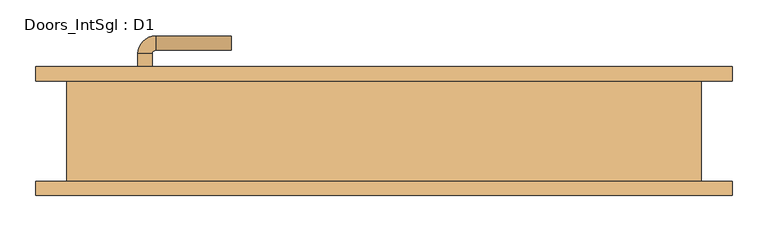
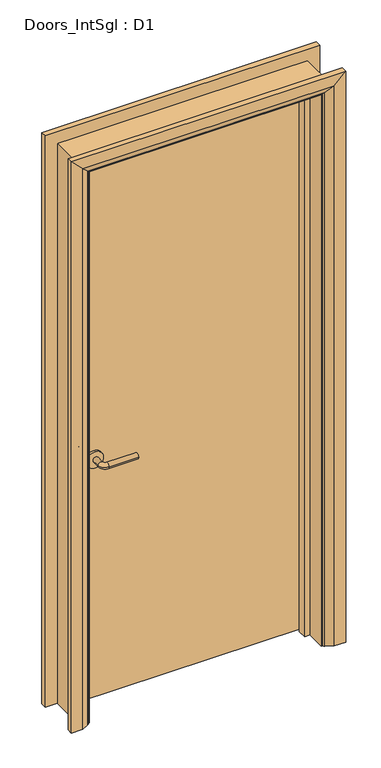
"""IFC4 building model written with IfcOpenShell, lengths in millimetres: door geometry, Doors_IntSgl : D1."""

from ifc_helpers import new_model, si_unit, point, frame, frame_2d, origin, place, context, project, spatial, polyline, circle_curve, ellipse_curve, trimmed, segment, composite_curve, outline, extrude, faceted_brep, source, transform, mapped, element, save
from ifc_brep_helpers import plane_surface, cylinder_surface, revolved_surface, advanced_brep


def doors_intsgl_d1_9c7e8c97(model_context):
    return source(origin(), model_context, "Body", "SolidModel", [
        advanced_brep(
        [(-343.0, 24.0, 900.0), (-323.0, 24.0, 900.0), (-323.0, -6.0, 900.0), (-343.0, -6.0, 900.0), (-318.0, -11.0, 900.0), (-318.0, -31.0, 900.0), (-213.0, -31.0, 900.0), (-213.0, -11.0, 900.0)],
        [
            (0, 1, circle_curve(frame((-333.0, 24.0, 900.0), z_axis=(0.0, 1.0, 0.0), x_axis=(1.0, 0.0, 0.0)), 10.0)),
            (1, 0, circle_curve(frame((-333.0, 24.0, 900.0), z_axis=(0.0, 1.0, 0.0), x_axis=(1.0, 0.0, 0.0)), 10.0)),
            (1, 2),
            (2, 3, circle_curve(frame((-333.0, -6.0, 900.0), z_axis=(0.0, 1.0, 0.0), x_axis=(1.0, 0.0, 0.0)), 10.0)),
            (3, 0),
            (3, 2, circle_curve(frame((-333.0, -6.0, 900.0), z_axis=(0.0, 1.0, 0.0), x_axis=(1.0, 0.0, 0.0)), 10.0)),
            (4, 5, circle_curve(frame((-318.0, -21.0, 900.0), z_axis=(-1.0, 0.0, 0.0), x_axis=(0.0, 1.0, 0.0)), 10.0)),
            (5, 3, circle_curve(frame((-318.0, -6.0, 900.0), z_axis=(0.0, 0.0, -1.0), x_axis=(-1.0, 0.0, 0.0)), 25.0)),
            (2, 4, circle_curve(frame((-318.0, -6.0, 900.0), z_axis=(0.0, 0.0, 1.0), x_axis=(-1.0, 0.0, 0.0)), 5.0)),
            (5, 4, circle_curve(frame((-318.0, -21.0, 900.0), z_axis=(-1.0, 0.0, 0.0), x_axis=(0.0, 1.0, 0.0)), 10.0)),
            (6, 7, circle_curve(frame((-213.0, -21.0, 900.0), z_axis=(1.0, 0.0, 0.0), x_axis=(0.0, 1.0, 0.0)), 10.0)),
            (7, 6, circle_curve(frame((-213.0, -21.0, 900.0), z_axis=(1.0, 0.0, 0.0), x_axis=(0.0, 1.0, 0.0)), 10.0)),
            (4, 7),
            (6, 5),
        ],
        [
            plane_surface(frame((-333.0, 24.0, 900.0), z_axis=(0.0, 1.0, 0.0), x_axis=(0.0, 0.0, 1.0))),
            cylinder_surface(frame((-333.0, 24.0, 900.0), z_axis=(0.0, 1.0, 0.0), x_axis=(1.0, 0.0, 0.0)), 10.0),
            revolved_surface(trimmed(ellipse_curve(frame((-333.0, -6.0, 900.0), z_axis=(0.0, -1.0, 0.0), x_axis=(1.0, 0.0, 0.0)), 10.0, 10.0), [point((-343.0, -6.0, 900.0))], [point((-323.0, -6.0, 900.0))], True, "CARTESIAN"), (-318.0, -6.0, 900.0), (0.0, 0.0, -1.0)),
            revolved_surface(trimmed(ellipse_curve(frame((-333.0, -6.0, 900.0), z_axis=(0.0, -1.0, 0.0), x_axis=(1.0, 0.0, 0.0)), 10.0, 10.0), [point((-323.0, -6.0, 900.0))], [point((-343.0, -6.0, 900.0))], True, "CARTESIAN"), (-318.0, -6.0, 900.0), (0.0, 0.0, -1.0)),
            plane_surface(frame((-213.0, -21.0, 900.0), z_axis=(1.0, 0.0, 0.0), x_axis=(0.0, 0.0, 1.0))),
            cylinder_surface(frame((-318.0, -21.0, 900.0), z_axis=(-1.0, 0.0, 0.0), x_axis=(0.0, 1.0, 0.0)), 10.0),
        ],
        [
            (0, [[1, 2]]),
            (1, [[3, 4, 5, -2]]),
            (1, [[-5, 6, -3, -1]]),
            (2, [[7, 8, -4, 9]]),
            (3, [[10, -9, -6, -8]]),
            (4, [[11, 12]]),
            (5, [[13, -11, 14, -7]]),
            (5, [[-14, -12, -13, -10]]),
        ],
    ),
        extrude(outline(composite_curve([segment(trimmed(circle_curve(frame_2d((900.0, -335.5)), 30.0), [point((900.0, -365.5))], [point((900.0, -305.5))], False, "CARTESIAN"), True, "CONTINUOUS"), segment(trimmed(circle_curve(frame_2d((900.0, -335.5)), 30.0), [point((900.0, -305.5))], [point((900.0, -365.5))], False, "CARTESIAN"), True, "CONTINUOUS")], self_intersect=False)), frame((0.0, 24.0, 0.0), z_axis=(0.0, 1.0, 0.0), x_axis=(0.0, 0.0, 1.0)), (0.0, 0.0, 1.0), 8.0),
        advanced_brep(
        [(-343.0, 78.0, 900.0), (-323.0, 78.0, 900.0), (-343.0, 108.0, 900.0), (-323.0, 108.0, 900.0), (-318.0, 113.0, 900.0), (-318.0, 133.0, 900.0), (-213.0, 133.0, 900.0), (-213.0, 113.0, 900.0)],
        [
            (0, 1, circle_curve(frame((-333.0, 78.0, 900.0), z_axis=(0.0, -1.0, 0.0), x_axis=(1.0, 0.0, 0.0)), 10.0)),
            (1, 0, circle_curve(frame((-333.0, 78.0, 900.0), z_axis=(0.0, -1.0, 0.0), x_axis=(1.0, 0.0, 0.0)), 10.0)),
            (0, 2),
            (2, 3, circle_curve(frame((-333.0, 108.0, 900.0), z_axis=(0.0, -1.0, 0.0), x_axis=(1.0, 0.0, 0.0)), 10.0)),
            (3, 1),
            (3, 2, circle_curve(frame((-333.0, 108.0, 900.0), z_axis=(0.0, -1.0, 0.0), x_axis=(1.0, 0.0, 0.0)), 10.0)),
            (4, 3, circle_curve(frame((-318.0, 108.0, 900.0), z_axis=(0.0, 0.0, 1.0), x_axis=(-1.0, 0.0, 0.0)), 5.0)),
            (2, 5, circle_curve(frame((-318.0, 108.0, 900.0), z_axis=(0.0, 0.0, -1.0), x_axis=(-1.0, 0.0, 0.0)), 25.0)),
            (5, 4, circle_curve(frame((-318.0, 123.0, 900.0), z_axis=(-1.0, 0.0, 0.0), x_axis=(0.0, -1.0, 0.0)), 10.0)),
            (4, 5, circle_curve(frame((-318.0, 123.0, 900.0), z_axis=(-1.0, 0.0, 0.0), x_axis=(0.0, -1.0, 0.0)), 10.0)),
            (6, 7, circle_curve(frame((-213.0, 123.0, 900.0), z_axis=(1.0, 0.0, 0.0), x_axis=(0.0, -1.0, 0.0)), 10.0)),
            (7, 6, circle_curve(frame((-213.0, 123.0, 900.0), z_axis=(1.0, 0.0, 0.0), x_axis=(0.0, -1.0, 0.0)), 10.0)),
            (5, 6),
            (7, 4),
        ],
        [
            plane_surface(frame((-333.0, 78.0, 900.0), z_axis=(0.0, -1.0, 0.0), x_axis=(0.0, 0.0, 1.0))),
            cylinder_surface(frame((-333.0, 78.0, 900.0), z_axis=(0.0, -1.0, 0.0), x_axis=(1.0, 0.0, 0.0)), 10.0),
            revolved_surface(trimmed(ellipse_curve(frame((-333.0, 108.0, 900.0), z_axis=(0.0, -1.0, 0.0), x_axis=(1.0, 0.0, 0.0)), 10.0, 10.0), [point((-343.0, 108.0, 900.0))], [point((-323.0, 108.0, 900.0))], True, "CARTESIAN"), (-318.0, 108.0, 900.0), (0.0, 0.0, -1.0)),
            revolved_surface(trimmed(ellipse_curve(frame((-333.0, 108.0, 900.0), z_axis=(0.0, -1.0, 0.0), x_axis=(1.0, 0.0, 0.0)), 10.0, 10.0), [point((-323.0, 108.0, 900.0))], [point((-343.0, 108.0, 900.0))], True, "CARTESIAN"), (-318.0, 108.0, 900.0), (0.0, 0.0, -1.0)),
            plane_surface(frame((-213.0, 123.0, 900.0), z_axis=(1.0, 0.0, 0.0), x_axis=(0.0, 0.0, 1.0))),
            cylinder_surface(frame((-318.0, 123.0, 900.0), z_axis=(-1.0, 0.0, 0.0), x_axis=(0.0, -1.0, 0.0)), 10.0),
        ],
        [
            (0, [[1, 2]]),
            (1, [[-1, 3, 4, 5]]),
            (1, [[-2, -5, 6, -3]]),
            (2, [[7, -4, 8, 9]]),
            (3, [[-8, -6, -7, 10]]),
            (4, [[11, 12]]),
            (5, [[-9, 13, -12, 14]]),
            (5, [[-10, -14, -11, -13]]),
        ],
    ),
        extrude(outline(composite_curve([segment(trimmed(circle_curve(frame_2d((900.0, -335.5)), 30.0), [point((900.0, -365.5))], [point((900.0, -305.5))], False, "CARTESIAN"), True, "CONTINUOUS"), segment(trimmed(circle_curve(frame_2d((900.0, -335.5)), 30.0), [point((900.0, -305.5))], [point((900.0, -365.5))], False, "CARTESIAN"), True, "CONTINUOUS")], self_intersect=False)), frame((0.0, 70.0, 0.0), z_axis=(0.0, 1.0, 0.0), x_axis=(0.0, 0.0, 1.0)), (0.0, 0.0, 1.0), 8.0),
        extrude(outline(polyline([(408.0, 32.0), (-408.0, 32.0), (-408.0, 70.0), (408.0, 70.0), (408.0, 32.0)])), frame((0.0, 0.0, 8.0), z_axis=(0.0, 0.0, 1.0), x_axis=(1.0, 0.0, 0.0)), (0.0, 0.0, 1.0), 2050.0),
        advanced_brep(
        [(485.0, 90.0, 0.0), (485.0, 70.0, 0.0), (415.0, 70.0, 0.0), (419.0, 76.0, 0.0), (445.0, 90.0, 0.0), (485.0, 90.0, 2135.0), (485.0, 70.0, 2135.0), (-485.0, 70.0, 2135.0), (-485.0, 70.0, 0.0), (-415.0, 70.0, 0.0), (-415.0, 70.0, 2065.0), (415.0, 70.0, 2065.0), (419.0, 76.0, 2069.0), (445.0, 90.0, 2095.0), (-445.0, 90.0, 2095.0), (-445.0, 90.0, 0.0), (-485.0, 90.0, 0.0), (-485.0, 90.0, 2135.0), (-419.0, 76.0, 0.0), (-419.0, 76.0, 2069.0)],
        [
            (0, 1),
            (1, 2),
            (2, 3, circle_curve(frame((423.0, 69.0, 0.0), z_axis=(0.0, 0.0, -1.0), x_axis=(1.0, 0.0, 0.0)), 8.0622577)),
            (3, 4),
            (4, 0),
            (0, 5),
            (5, 6),
            (6, 1),
            (6, 7),
            (7, 8),
            (8, 9),
            (9, 10),
            (10, 11),
            (11, 2),
            (11, 12, ellipse_curve(frame((423.0, 69.0, 2073.0), z_axis=(0.7071067811865475, 0.0, -0.7071067811865475), x_axis=(-0.7071067811865474, 0.0, -0.7071067811865476)), 11.4017543, 8.0622577)),
            (12, 3),
            (12, 13),
            (13, 4),
            (13, 14),
            (14, 15),
            (15, 16),
            (16, 17),
            (17, 5),
            (7, 17),
            (16, 8),
            (15, 18),
            (18, 9, circle_curve(frame((-423.0, 69.0, 0.0), z_axis=(0.0, 0.0, -1.0), x_axis=(-1.0, 0.0, 0.0)), 8.0622577)),
            (19, 10, ellipse_curve(frame((-423.0, 69.0, 2073.0), z_axis=(-0.7071067811865475, 0.0, -0.7071067811865475), x_axis=(-0.7071067811865474, 0.0, 0.7071067811865476)), 11.4017543, 8.0622577)),
            (18, 19),
            (14, 19),
            (19, 12),
        ],
        [
            plane_surface(frame((415.0, 70.0, 0.0), z_axis=(0.0, 0.0, -1.0), x_axis=(0.0, -1.0, 0.0))),
            plane_surface(frame((485.0, 90.0, 0.0), z_axis=(1.0, 0.0, 0.0), x_axis=(0.0, 0.0, 1.0))),
            plane_surface(frame((485.0, 70.0, 0.0), z_axis=(0.0, -1.0, 0.0), x_axis=(0.0, 0.0, 1.0))),
            cylinder_surface(frame((423.0, 69.0, 0.0), z_axis=(0.0, 0.0, -1.0), x_axis=(1.0, 0.0, 0.0)), 8.0622577),
            plane_surface(frame((419.0, 76.0, 0.0), z_axis=(-0.4740998230350126, 0.880471099922178, 0.0), x_axis=(0.0, 0.0, 1.0))),
            plane_surface(frame((445.0, 90.0, 0.0), z_axis=(0.0, 1.0, 0.0), x_axis=(0.0, 0.0, 1.0))),
            plane_surface(frame((-485.0, 90.0, 2135.0), z_axis=(-1.0, 0.0, 0.0), x_axis=(0.0, 0.0, -1.0))),
            plane_surface(frame((-415.0, 70.0, 0.0), z_axis=(0.0, 0.0, -1.0), x_axis=(0.0, -1.0, 0.0))),
            cylinder_surface(frame((-423.0, 69.0, 2065.0), z_axis=(0.0, 0.0, 1.0), x_axis=(-1.0, 0.0, 0.0)), 8.0622577),
            plane_surface(frame((-419.0, 76.0, 2069.0), z_axis=(0.47409982303501824, 0.8804710999221749, 0.0), x_axis=(0.0, 0.0, -1.0))),
            plane_surface(frame((485.0, 90.0, 2135.0), z_axis=(0.0, 0.0, 1.0), x_axis=(-1.0, 0.0, 0.0))),
            cylinder_surface(frame((415.0, 69.0, 2073.0), z_axis=(1.0, 0.0, 0.0), x_axis=(0.0, 0.0, 1.0)), 8.0622577),
            plane_surface(frame((419.0, 76.0, 2069.0), z_axis=(0.0, 0.8804710999221764, -0.4740998230350154), x_axis=(-1.0, 0.0, 0.0))),
        ],
        [
            (0, [[1, 2, 3, 4, 5]]),
            (1, [[-1, 6, 7, 8]]),
            (2, [[-2, -8, 9, 10, 11, 12, 13, 14]]),
            (3, [[-3, -14, 15, 16]]),
            (4, [[-4, -16, 17, 18]]),
            (5, [[-5, -18, 19, 20, 21, 22, 23, -6]]),
            (6, [[24, -22, 25, -10]]),
            (7, [[-21, 26, 27, -11, -25]]),
            (8, [[28, -12, -27, 29]]),
            (9, [[30, -29, -26, -20]]),
            (10, [[-7, -23, -24, -9]]),
            (11, [[-15, -13, -28, 31]]),
            (12, [[-17, -31, -30, -19]]),
        ],
    ),
        extrude(outline(polyline([(0.0, -410.0), (0.0, -391.0), (2041.0, -391.0), (2041.0, 391.0), (0.0, 391.0), (0.0, 410.0), (2060.0, 410.0), (2060.0, -410.0), (0.0, -410.0)])), frame((0.0, -2.0, 0.0), z_axis=(0.0, 1.0, 0.0), x_axis=(0.0, 0.0, 1.0)), (0.0, 0.0, 1.0), 32.0),
        advanced_brep(
        [(-485.0, -90.0, 0.0), (-485.0, -70.0, 0.0), (-415.0, -70.0, 0.0), (-419.0, -76.0, 0.0), (-445.0, -90.0, 0.0), (-485.0, -90.0, 2135.0), (-485.0, -70.0, 2135.0), (-415.0, -70.0, 2065.0), (-419.0, -76.0, 2069.0), (-445.0, -90.0, 2095.0), (485.0, -90.0, 0.0), (445.0, -90.0, 0.0), (419.0, -76.0, 0.0), (415.0, -70.0, 0.0), (485.0, -70.0, 0.0), (485.0, -90.0, 2135.0), (445.0, -90.0, 2095.0), (419.0, -76.0, 2069.0), (415.0, -70.0, 2065.0), (485.0, -70.0, 2135.0)],
        [
            (0, 1),
            (1, 2),
            (2, 3, circle_curve(frame((-423.0, -69.0, 0.0), z_axis=(0.0, 0.0, -1.0), x_axis=(-1.0, 0.0, 0.0)), 8.0622577)),
            (3, 4),
            (4, 0),
            (0, 5),
            (5, 6),
            (6, 1),
            (6, 7),
            (7, 2),
            (7, 8, ellipse_curve(frame((-423.0, -69.0, 2073.0), z_axis=(-0.7071067811865475, 0.0, -0.7071067811865475), x_axis=(0.7071067811865474, 0.0, -0.7071067811865476)), 11.4017543, 8.0622577)),
            (8, 3),
            (8, 9),
            (9, 4),
            (9, 5),
            (10, 11),
            (11, 12),
            (12, 13, circle_curve(frame((423.0, -69.0, 0.0), z_axis=(0.0, 0.0, -1.0), x_axis=(1.0, 0.0, 0.0)), 8.0622577)),
            (13, 14),
            (14, 10),
            (15, 16),
            (16, 11),
            (10, 15),
            (16, 17),
            (17, 12),
            (17, 18, ellipse_curve(frame((423.0, -69.0, 2073.0), z_axis=(0.7071067811865475, 0.0, -0.7071067811865475), x_axis=(0.7071067811865474, 0.0, 0.7071067811865476)), 11.4017543, 8.0622577)),
            (18, 13),
            (18, 19),
            (19, 14),
            (19, 15),
            (5, 15),
            (19, 6),
            (18, 7),
            (17, 8),
            (16, 9),
        ],
        [
            plane_surface(frame((-415.0, -142.8010989, 0.0), z_axis=(0.0, 0.0, -1.0), x_axis=(1.0, 0.0, 0.0))),
            plane_surface(frame((-485.0, -90.0, 0.0), z_axis=(-1.0, 0.0, 0.0), x_axis=(0.0, 0.0, 1.0))),
            plane_surface(frame((-485.0, -70.0, 0.0), z_axis=(0.0, 1.0, 0.0), x_axis=(0.0, 0.0, 1.0))),
            cylinder_surface(frame((-423.0, -69.0, 0.0), z_axis=(0.0, 0.0, -1.0), x_axis=(-1.0, 0.0, 0.0)), 8.0622577),
            plane_surface(frame((-419.0, -76.0, 0.0), z_axis=(0.4740998230350183, -0.8804710999221749, 0.0), x_axis=(0.0, 0.0, 1.0))),
            plane_surface(frame((-445.0, -90.0, 0.0), z_axis=(0.0, -1.0, 0.0), x_axis=(0.0, 0.0, 1.0))),
            plane_surface(frame((415.0, -142.8010989, 0.0), z_axis=(0.0, 0.0, -1.0), x_axis=(-1.0, 0.0, 0.0))),
            plane_surface(frame((445.0, -90.0, 2095.0), z_axis=(0.0, -1.0, 0.0), x_axis=(0.0, 0.0, -1.0))),
            plane_surface(frame((419.0, -76.0, 2069.0), z_axis=(-0.4740998230350183, -0.8804710999221749, 0.0), x_axis=(0.0, 0.0, -1.0))),
            cylinder_surface(frame((423.0, -69.0, 2065.0), z_axis=(0.0, 0.0, 1.0), x_axis=(1.0, 0.0, 0.0)), 8.0622577),
            plane_surface(frame((485.0, -70.0, 2135.0), z_axis=(0.0, 1.0, 0.0), x_axis=(0.0, 0.0, -1.0))),
            plane_surface(frame((485.0, -90.0, 2135.0), z_axis=(1.0, 0.0, 0.0), x_axis=(0.0, 0.0, -1.0))),
            plane_surface(frame((-485.0, -90.0, 2135.0), z_axis=(0.0, 0.0, 1.0), x_axis=(1.0, 0.0, 0.0))),
            plane_surface(frame((-485.0, -70.0, 2135.0), z_axis=(0.0, 1.0, 0.0), x_axis=(1.0, 0.0, 0.0))),
            cylinder_surface(frame((-415.0, -69.0, 2073.0), z_axis=(-1.0, 0.0, 0.0), x_axis=(0.0, 0.0, 1.0)), 8.0622577),
            plane_surface(frame((-419.0, -76.0, 2069.0), z_axis=(0.0, -0.8804710999221749, -0.4740998230350183), x_axis=(1.0, 0.0, 0.0))),
            plane_surface(frame((-445.0, -90.0, 2095.0), z_axis=(0.0, -1.0, 0.0), x_axis=(1.0, 0.0, 0.0))),
        ],
        [
            (0, [[1, 2, 3, 4, 5]]),
            (1, [[-1, 6, 7, 8]]),
            (2, [[-2, -8, 9, 10]]),
            (3, [[-3, -10, 11, 12]]),
            (4, [[-4, -12, 13, 14]]),
            (5, [[-5, -14, 15, -6]]),
            (6, [[16, 17, 18, 19, 20]]),
            (7, [[21, 22, -16, 23]]),
            (8, [[24, 25, -17, -22]]),
            (9, [[26, 27, -18, -25]]),
            (10, [[28, 29, -19, -27]]),
            (11, [[30, -23, -20, -29]]),
            (12, [[-7, 31, -30, 32]]),
            (13, [[-9, -32, -28, 33]]),
            (14, [[-11, -33, -26, 34]]),
            (15, [[-13, -34, -24, 35]]),
            (16, [[-15, -35, -21, -31]]),
        ],
    ),
        faceted_brep([(-410.0, 70.0, 0.0), (-410.0, -70.0, 0.0), (-442.0, -70.0, 0.0), (-442.0, 70.0, 0.0), (-410.0, 70.0, 2060.0), (-410.0, -70.0, 2060.0), (-442.0, -70.0, 2092.0), (-442.0, 70.0, 2092.0), (410.0, 70.0, 0.0), (442.0, 70.0, 0.0), (442.0, -70.0, 0.0), (410.0, -70.0, 0.0), (410.0, 70.0, 2060.0), (442.0, 70.0, 2092.0), (442.0, -70.0, 2092.0), (410.0, -70.0, 2060.0)], [[[0, 1, 2, 3]], [[1, 0, 4, 5]], [[2, 1, 5, 6]], [[3, 2, 6, 7]], [[0, 3, 7, 4]], [[8, 9, 10, 11]], [[12, 13, 9, 8]], [[13, 14, 10, 9]], [[14, 15, 11, 10]], [[15, 12, 8, 11]], [[5, 4, 12, 15]], [[6, 5, 15, 14]], [[7, 6, 14, 13]], [[4, 7, 13, 12]]]),
    ])


if __name__ == "__main__":
    model = new_model("IFC4")
    model_context = context("Model", 3, world=origin())
    ifc_project = project(units=[si_unit("LENGTHUNIT", "METRE", prefix="MILLI")], contexts=[model_context])
    site = spatial("IfcSite", under=ifc_project)
    building = spatial("IfcBuilding", under=site)
    placement = place(None, origin())
    doors_intsgl_d1_shape = doors_intsgl_d1_9c7e8c97(model_context)
    element("IfcDoor", 1, ObjectType="Doors_IntSgl : D1", at=placement, inside=building, context=model_context, shape_type="MappedRepresentation", body=[
        mapped(doors_intsgl_d1_shape, transform((0.0, 0.0, 0.0), x_axis=(1.0, 0.0, 0.0), y_axis=(0.0, 1.0, 0.0), z_axis=(0.0, 0.0, 1.0))),
    ])
    save(model, "model.ifc")

# Revit data of these elements
# Type "Doors_IntSgl : D1"
#   Type Mark = "46"
#   Type Comments = "Internal Single"
#   Operation = "SingleSwingRight"
#   Manufacturer = "Revit"
#   Keynote = "L20"
#   Description = "Internal Single Door"
#   Analytic Construction = "Metal"
#   UnderCut = 8 mm
#   Tolerance = 2 mm
#   Thickness = 38 mm
#   Thermal Resistance (R) = 0.270117 (m²·K)/W
#   Structural Tolerance = 8 mm
#   StopDepth = 32 mm
#   Stop Thickness = 19 mm
#   Rough Width = 900 mm
#   Rough Height = 2100 mm
#   Height to Top Lock Rail = 1000 mm
#   Heat Transfer Coefficient (U) = 3.7021 W/(m²·K)
#   Handle Z Distance = 900 mm
#   Handle X Distance = 75 mm
#   Frame Thickness = 32 mm
#   Door Panel Width = 816 mm
#   Door Panel Thickness = 38 mm
#   Door Panel Offset = 0 mm
#   Height = 2100 mm
#   Width = 900 mm
#   Door Panel Height = 2050 mm
#   Architrave Setback = 5 mm
#   Vis - Ironmongery = yes
#   Material Ironmongery = Door - Handle
#   Material Frame = Door - Frame/Mullion (1)
#   Material Door = Door - Panel
#   Material Architrave = Door - Architrave
#   Visual Light Transmittance = 0
#   Solar Heat Gain Coefficient = 0
#   Function = (empty or 0)
#   Wall Closure = (empty or 0)
# Element 1 (IfcDoor, "Doors_IntSgl : D1")
#   Materials on its faces: "Door - Architrave", "Door - Handle", "Door - Frame/Mullion (1)", "Door - Panel"
# Materials
#   "Door - Handle": colour RGB 0 0 0, transparency 0, Keynote = "P21", Cost = 0
#   "Door - Frame/Mullion (1)": class "Wood", colour RGB 212 179 113, transparency 0, Keynote = "L20", Cost = 0
#   "Door - Panel": class "Wood", colour RGB 210 159 95, transparency 0, Keynote = "L20", Cost = 0
#   "Door - Architrave": class "Wood", colour RGB 154 90 5, transparency 0, Keynote = "P20", Cost = 0
